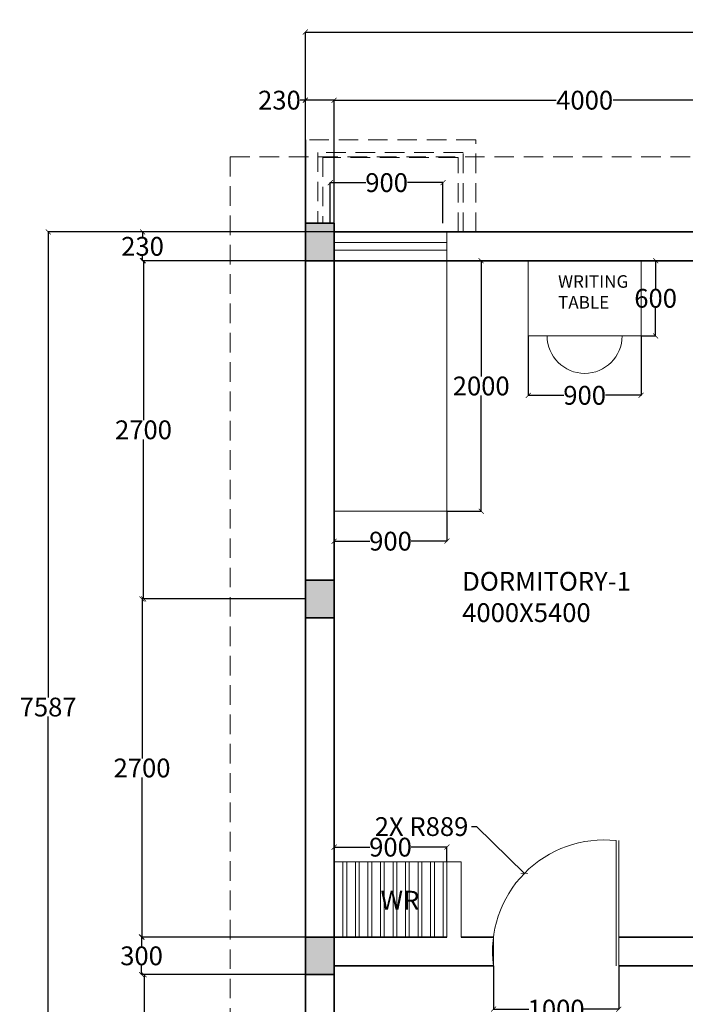
# Model space of a CAD drawing. Units: millimetres. Extents: x 32888 to 53184, y 27889 to 39696.
# Tile 2 of 6: x 32888 to 38202, y 31834 to 39696. Entities that reach past the tile are written whole.
import ezdxf

# ---------------------------------------------------------------- set-up
doc = ezdxf.new("R2010")
doc.units = ezdxf.units.MM
doc.header["$LTSCALE"] = 50
doc.header["$MEASUREMENT"] = 0
doc.linetypes.add('HIDDEN2', pattern=[0.1875, 0.125, -0.0625])
for name, color, linetype, lineweight in [('A-ANNO-DIMS', 2, 'Continuous', 18), ('A-ANNO-TEXT', 7, 'Continuous', 18), ('A-AREA-IDEN', 7, 'Continuous', 18), ('A-COLS', 1, 'Continuous', 35), ('A-COLS-PATT', 18, 'Continuous', 18), ('A-DOOR', 4, 'Continuous', 18), ('A-DOOR-HIDN', 4, 'HIDDEN2', 18), ('A-FURN', 8, 'Continuous', 18), ('A-FURN-CASE', 8, 'Continuous', 18), ('A-GLAZ', 4, 'Continuous', 18), ('A-ROOF-OVHD', 8, 'HIDDEN2', 18), ('A-WALL', 7, 'Continuous', 35)]:
    doc.layers.add(name, color=color, linetype=linetype, lineweight=lineweight)
doc.styles.get("Standard").update_dxf_attribs({"font": 'arial.ttf'})
doc.dimstyles.get("Standard").update_dxf_attribs({"dimtxt": 150, "dimasz": 40, "dimexe": 0.18, "dimexo": 0.0625, "dimgap": 0.09, "dimtad": 0, "dimtih": 1, "dimtoh": 1, "dimdec": 0, "dimzin": 0, "dimdsep": 46, "dimtxsty": 'Standard', "dimblk": 'ARCHTICK', "dimcen": 0, "dimadec": 0, "dimazin": 0, "dimtfac": 1, "dimtdec": 0, "dimtofl": 0, "dimtmove": 0, "dimatfit": 3, "dimldrblk": 'ARCHTICK', "dimfxl": 1, "dimtolj": 1, "dimtzin": 0, "dimarcsym": 1})

# ---------------------------------------------------------------- blocks, each defined once
blk = doc.blocks.new('_ArchTick')
at = {"color": 0, "linetype": 'ByBlock', "const_width": 0.15}
blk.add_lwpolyline([(-0.5, -0.5), (0.5, 0.5)], dxfattribs=at)
blk = doc.blocks.new('*D15')
at = {"layer": 'A-ANNO-DIMS', "color": 0, "lineweight": -2, "ltscale": 50, "transparency": 16777216}
for p, q in [((35398.9, 32971.1), (35398.9, 33089.1)), ((35398.9, 33088.9), (35683.4, 33088.9)), ((36298.9, 33088.9), (36014.5, 33088.9)), ((36298.9, 32971.1), (36298.9, 33089.1))]:
    blk.add_line(p, q, dxfattribs=at)
at = {"layer": 'Defpoints', "color": 0, "ltscale": 50, "transparency": 16777216}
for p in [(36298.9, 33088.9), (35398.9, 32971), (36298.9, 32971)]:
    blk.add_point(p, dxfattribs=at)
at = {"layer": 'A-ANNO-DIMS', "color": 0, "lineweight": -2, "ltscale": 50, "transparency": 16777216, "xscale": 40, "yscale": 40, "zscale": 40, "rotation": 180}
blk.add_blockref('_ArchTick', (35398.9, 33088.9), dxfattribs=at)
at = {"layer": 'A-ANNO-DIMS', "color": 0, "lineweight": -2, "ltscale": 50, "transparency": 16777216, "xscale": 40, "yscale": 40, "zscale": 40}
blk.add_blockref('_ArchTick', (36298.9, 33088.9), dxfattribs=at)
at = {"layer": 'A-ANNO-DIMS', "color": 0, "ltscale": 50, "transparency": 16777216, "insert": (35848.9, 33088.9), "char_height": 150, "attachment_point": 5}
blk.add_mtext('\\A1;900', dxfattribs=at)
blk = doc.blocks.new('*D16')
at = {"layer": 'A-ANNO-DIMS', "color": 0, "lineweight": -2, "ltscale": 50, "transparency": 16777216}
for p, q in [((36671.2, 32140.9), (36671.2, 31795.5)), ((37671.2, 32140.9), (37671.2, 31795.5)), ((36671.2, 31795.7), (36954.5, 31795.7)), ((37671.2, 31795.7), (37388, 31795.7))]:
    blk.add_line(p, q, dxfattribs=at)
at = {"layer": 'Defpoints', "color": 0, "ltscale": 50, "transparency": 16777216}
for p in [(36671.2, 32141), (37671.2, 32141), (37671.2, 31795.7)]:
    blk.add_point(p, dxfattribs=at)
at = {"layer": 'A-ANNO-DIMS', "color": 0, "lineweight": -2, "ltscale": 50, "transparency": 16777216, "xscale": 40, "yscale": 40, "zscale": 40, "rotation": 180}
blk.add_blockref('_ArchTick', (36671.2, 31795.7), dxfattribs=at)
at = {"layer": 'A-ANNO-DIMS', "color": 0, "lineweight": -2, "ltscale": 50, "transparency": 16777216, "xscale": 40, "yscale": 40, "zscale": 40}
blk.add_blockref('_ArchTick', (37671.2, 31795.7), dxfattribs=at)
at = {"layer": 'A-ANNO-DIMS', "color": 0, "ltscale": 50, "transparency": 16777216, "insert": (37171.2, 31795.7), "char_height": 150, "attachment_point": 5}
blk.add_mtext('\\A1;1000', dxfattribs=at)
blk = doc.blocks.new('*D22')
at = {"layer": 'A-ANNO-DIMS', "color": 0, "lineweight": -2, "ltscale": 50, "transparency": 16777216}
for p, q in [((35168.9, 32071), (33881.1, 32071)), ((33881.3, 32071), (33881.3, 31247.7)), ((33881.3, 30271), (33881.3, 31094.3)), ((35168.9, 30271), (33881.1, 30271))]:
    blk.add_line(p, q, dxfattribs=at)
at = {"layer": 'Defpoints', "color": 0, "ltscale": 50, "transparency": 16777216}
for p in [(35168.9, 32071), (33881.3, 30271), (35168.9, 30271)]:
    blk.add_point(p, dxfattribs=at)
at = {"layer": 'A-ANNO-DIMS', "color": 0, "lineweight": -2, "ltscale": 50, "transparency": 16777216, "xscale": 40, "yscale": 40, "zscale": 40}
for p, rotation in [((33881.3, 32071), 90), ((33881.3, 30271), 270)]:
    blk.add_blockref('_ArchTick', p, dxfattribs=dict(at, rotation=rotation))
at = {"layer": 'A-ANNO-DIMS', "color": 0, "ltscale": 50, "transparency": 16777216, "insert": (33881.3, 31171), "char_height": 150, "attachment_point": 5}
blk.add_mtext('\\A1;1800', dxfattribs=at)
blk = doc.blocks.new('*D23')
at = {"layer": 'A-ANNO-DIMS', "color": 0, "lineweight": -2, "ltscale": 50, "transparency": 16777216}
for p, q in [((35168.9, 32371), (33861.1, 32371)), ((33861.3, 32371), (33861.3, 32297.7)), ((33861.3, 32071), (33861.3, 32144.3)), ((35168.9, 32071), (33861.1, 32071))]:
    blk.add_line(p, q, dxfattribs=at)
at = {"layer": 'Defpoints', "color": 0, "ltscale": 50, "transparency": 16777216}
for p in [(33861.3, 32371), (35168.9, 32371), (35168.9, 32071)]:
    blk.add_point(p, dxfattribs=at)
at = {"layer": 'A-ANNO-DIMS', "color": 0, "lineweight": -2, "ltscale": 50, "transparency": 16777216, "xscale": 40, "yscale": 40, "zscale": 40}
for p, rotation in [((33861.3, 32371), 90), ((33861.3, 32071), 270)]:
    blk.add_blockref('_ArchTick', p, dxfattribs=dict(at, rotation=rotation))
at = {"layer": 'A-ANNO-DIMS', "color": 0, "ltscale": 50, "transparency": 16777216, "insert": (33861.3, 32221), "char_height": 150, "attachment_point": 5}
blk.add_mtext('\\A1;300', dxfattribs=at)
blk = doc.blocks.new('*D24')
at = {"layer": 'A-ANNO-DIMS', "color": 0, "lineweight": -2, "ltscale": 50, "transparency": 16777216}
for p, q in [((35168.9, 35071), (33864.9, 35071)), ((33865.1, 35071), (33865.1, 33797.7)), ((33865.1, 32371), (33865.1, 33644.3)), ((35168.9, 32371), (33864.9, 32371))]:
    blk.add_line(p, q, dxfattribs=at)
at = {"layer": 'Defpoints', "color": 0, "ltscale": 50, "transparency": 16777216}
for p in [(33865.1, 35071), (35168.9, 35071), (35168.9, 32371)]:
    blk.add_point(p, dxfattribs=at)
at = {"layer": 'A-ANNO-DIMS', "color": 0, "lineweight": -2, "ltscale": 50, "transparency": 16777216, "xscale": 40, "yscale": 40, "zscale": 40}
for p, rotation in [((33865.1, 35071), 90), ((33865.1, 32371), 270)]:
    blk.add_blockref('_ArchTick', p, dxfattribs=dict(at, rotation=rotation))
at = {"layer": 'A-ANNO-DIMS', "color": 0, "ltscale": 50, "transparency": 16777216, "insert": (33865.1, 33721), "char_height": 150, "attachment_point": 5}
blk.add_mtext('\\A1;2700', dxfattribs=at)
blk = doc.blocks.new('*D25')
at = {"layer": 'A-ANNO-DIMS', "color": 0, "lineweight": -2, "ltscale": 50, "transparency": 16777216}
for p, q in [((35168.9, 37771), (33876.5, 37771)), ((33876.7, 37771), (33876.7, 36497.7)), ((33876.7, 35071), (33876.7, 36344.3)), ((35168.9, 35071), (33876.5, 35071))]:
    blk.add_line(p, q, dxfattribs=at)
at = {"layer": 'Defpoints', "color": 0, "ltscale": 50, "transparency": 16777216}
for p in [(33876.7, 37771), (35168.9, 37771), (35168.9, 35071)]:
    blk.add_point(p, dxfattribs=at)
at = {"layer": 'A-ANNO-DIMS', "color": 0, "lineweight": -2, "ltscale": 50, "transparency": 16777216, "xscale": 40, "yscale": 40, "zscale": 40}
for p, rotation in [((33876.7, 37771), 90), ((33876.7, 35071), 270)]:
    blk.add_blockref('_ArchTick', p, dxfattribs=dict(at, rotation=rotation))
at = {"layer": 'A-ANNO-DIMS', "color": 0, "ltscale": 50, "transparency": 16777216, "insert": (33876.7, 36421), "char_height": 150, "attachment_point": 5}
blk.add_mtext('\\A1;2700', dxfattribs=at)
blk = doc.blocks.new('*D26')
at = {"layer": 'A-ANNO-DIMS', "color": 0, "lineweight": -2, "ltscale": 50, "transparency": 16777216}
for p, q in [((35398.9, 38001), (33869, 38001)), ((33869.2, 38001), (33869.2, 37962.7)), ((35398.9, 37771), (33869, 37771)), ((33869.2, 37771), (33869.2, 37809.3))]:
    blk.add_line(p, q, dxfattribs=at)
at = {"layer": 'Defpoints', "color": 0, "ltscale": 50, "transparency": 16777216}
for p in [(33869.2, 38001), (35398.9, 38001), (35398.9, 37771)]:
    blk.add_point(p, dxfattribs=at)
at = {"layer": 'A-ANNO-DIMS', "color": 0, "lineweight": -2, "ltscale": 50, "transparency": 16777216, "xscale": 40, "yscale": 40, "zscale": 40}
for p, rotation in [((33869.2, 38001), 90), ((33869.2, 37771), 270)]:
    blk.add_blockref('_ArchTick', p, dxfattribs=dict(at, rotation=rotation))
at = {"layer": 'A-ANNO-DIMS', "color": 0, "ltscale": 50, "transparency": 16777216, "insert": (33869.2, 37886), "char_height": 150, "attachment_point": 5}
blk.add_mtext('\\A1;230', dxfattribs=at)
blk = doc.blocks.new('*D39')
at = {"layer": 'A-ANNO-DIMS', "color": 0, "lineweight": -2, "ltscale": 50, "transparency": 16777216}
for p, q in [((36948.9, 37170.9), (36948.9, 36696.3)), ((37848.9, 37170.9), (37848.9, 36696.3)), ((36948.9, 36696.4), (37233.4, 36696.4)), ((37848.9, 36696.4), (37564.5, 36696.4))]:
    blk.add_line(p, q, dxfattribs=at)
at = {"layer": 'Defpoints', "color": 0, "ltscale": 50, "transparency": 16777216}
for p in [(36948.9, 37171), (37848.9, 37171), (36948.9, 36696.4)]:
    blk.add_point(p, dxfattribs=at)
at = {"layer": 'A-ANNO-DIMS', "color": 0, "lineweight": -2, "ltscale": 50, "transparency": 16777216, "xscale": 40, "yscale": 40, "zscale": 40, "rotation": 180}
blk.add_blockref('_ArchTick', (36948.9, 36696.4), dxfattribs=at)
at = {"layer": 'A-ANNO-DIMS', "color": 0, "lineweight": -2, "ltscale": 50, "transparency": 16777216, "xscale": 40, "yscale": 40, "zscale": 40}
blk.add_blockref('_ArchTick', (37848.9, 36696.4), dxfattribs=at)
at = {"layer": 'A-ANNO-DIMS', "color": 0, "ltscale": 50, "transparency": 16777216, "insert": (37398.9, 36696.4), "char_height": 150, "attachment_point": 5}
blk.add_mtext('\\A1;900', dxfattribs=at)
blk = doc.blocks.new('*D40')
at = {"layer": 'A-ANNO-DIMS', "color": 0, "lineweight": -2, "ltscale": 50, "transparency": 16777216}
for p, q in [((37849, 37771), (37965.7, 37771)), ((37965.6, 37771), (37965.6, 37547.7)), ((37965.6, 37171), (37965.6, 37394.3)), ((37849, 37171), (37965.7, 37171))]:
    blk.add_line(p, q, dxfattribs=at)
at = {"layer": 'Defpoints', "color": 0, "ltscale": 50, "transparency": 16777216}
for p in [(37848.9, 37771), (37965.6, 37771), (37848.9, 37171)]:
    blk.add_point(p, dxfattribs=at)
at = {"layer": 'A-ANNO-DIMS', "color": 0, "lineweight": -2, "ltscale": 50, "transparency": 16777216, "xscale": 40, "yscale": 40, "zscale": 40}
for p, rotation in [((37965.6, 37771), 90), ((37965.6, 37171), 270)]:
    blk.add_blockref('_ArchTick', p, dxfattribs=dict(at, rotation=rotation))
at = {"layer": 'A-ANNO-DIMS', "color": 0, "ltscale": 50, "transparency": 16777216, "insert": (37965.6, 37471), "char_height": 150, "attachment_point": 5}
blk.add_mtext('\\A1;600', dxfattribs=at)
blk = doc.blocks.new('*D41')
at = {"layer": 'A-ANNO-DIMS', "color": 0, "lineweight": -2, "ltscale": 50, "transparency": 16777216}
for p, q in [((36299, 37771), (36573.1, 37771)), ((36572.9, 37771), (36572.9, 36847.7)), ((36572.9, 35771), (36572.9, 36694.3)), ((36299, 35771), (36573.1, 35771))]:
    blk.add_line(p, q, dxfattribs=at)
at = {"layer": 'Defpoints', "color": 0, "ltscale": 50, "transparency": 16777216}
for p in [(36298.9, 37771), (36572.9, 37771), (36298.9, 35771)]:
    blk.add_point(p, dxfattribs=at)
at = {"layer": 'A-ANNO-DIMS', "color": 0, "lineweight": -2, "ltscale": 50, "transparency": 16777216, "xscale": 40, "yscale": 40, "zscale": 40}
for p, rotation in [((36572.9, 37771), 90), ((36572.9, 35771), 270)]:
    blk.add_blockref('_ArchTick', p, dxfattribs=dict(at, rotation=rotation))
at = {"layer": 'A-ANNO-DIMS', "color": 0, "ltscale": 50, "transparency": 16777216, "insert": (36572.9, 36771), "char_height": 150, "attachment_point": 5}
blk.add_mtext('\\A1;2000', dxfattribs=at)
blk = doc.blocks.new('*D42')
at = {"layer": 'A-ANNO-DIMS', "color": 0, "lineweight": -2, "ltscale": 50, "transparency": 16777216}
for p, q in [((35398.9, 35770.9), (35398.9, 35531.8)), ((36298.9, 35770.9), (36298.9, 35531.8)), ((35398.9, 35531.9), (35683.4, 35531.9)), ((36298.9, 35531.9), (36014.5, 35531.9))]:
    blk.add_line(p, q, dxfattribs=at)
at = {"layer": 'Defpoints', "color": 0, "ltscale": 50, "transparency": 16777216}
for p in [(35398.9, 35771), (36298.9, 35771), (35398.9, 35531.9)]:
    blk.add_point(p, dxfattribs=at)
at = {"layer": 'A-ANNO-DIMS', "color": 0, "lineweight": -2, "ltscale": 50, "transparency": 16777216, "xscale": 40, "yscale": 40, "zscale": 40, "rotation": 180}
blk.add_blockref('_ArchTick', (35398.9, 35531.9), dxfattribs=at)
at = {"layer": 'A-ANNO-DIMS', "color": 0, "lineweight": -2, "ltscale": 50, "transparency": 16777216, "xscale": 40, "yscale": 40, "zscale": 40}
blk.add_blockref('_ArchTick', (36298.9, 35531.9), dxfattribs=at)
at = {"layer": 'A-ANNO-DIMS', "color": 0, "ltscale": 50, "transparency": 16777216, "insert": (35848.9, 35531.9), "char_height": 150, "attachment_point": 5}
blk.add_mtext('\\A1;900', dxfattribs=at)
blk = doc.blocks.new('*D47')
at = {"layer": 'A-ANNO-DIMS', "color": 0, "lineweight": -2, "ltscale": 50, "transparency": 16777216}
for p, q in [((35367.9, 38071.1), (35367.9, 38395)), ((35367.9, 38394.8), (35652.4, 38394.8)), ((36267.9, 38394.8), (35983.5, 38394.8)), ((36267.9, 38071.1), (36267.9, 38395))]:
    blk.add_line(p, q, dxfattribs=at)
at = {"layer": 'Defpoints', "color": 0, "ltscale": 50, "transparency": 16777216}
for p in [(36267.9, 38394.8), (35367.9, 38071), (36267.9, 38071)]:
    blk.add_point(p, dxfattribs=at)
at = {"layer": 'A-ANNO-DIMS', "color": 0, "lineweight": -2, "ltscale": 50, "transparency": 16777216, "xscale": 40, "yscale": 40, "zscale": 40, "rotation": 180}
blk.add_blockref('_ArchTick', (35367.9, 38394.8), dxfattribs=at)
at = {"layer": 'A-ANNO-DIMS', "color": 0, "lineweight": -2, "ltscale": 50, "transparency": 16777216, "xscale": 40, "yscale": 40, "zscale": 40}
blk.add_blockref('_ArchTick', (36267.9, 38394.8), dxfattribs=at)
at = {"layer": 'A-ANNO-DIMS', "color": 0, "ltscale": 50, "transparency": 16777216, "insert": (35817.9, 38394.8), "char_height": 150, "attachment_point": 5}
blk.add_mtext('\\A1;900', dxfattribs=at)
blk = doc.blocks.new('*D54')
at = {"layer": 'A-ANNO-DIMS', "color": 0, "lineweight": -2, "ltscale": 50, "transparency": 16777216}
for p, q in [((35398.9, 38001.1), (35398.9, 39053.1)), ((35398.9, 39052.9), (37172.1, 39052.9)), ((39398.9, 39052.9), (37625.8, 39052.9)), ((39398.9, 38001.1), (39398.9, 39053.1))]:
    blk.add_line(p, q, dxfattribs=at)
at = {"layer": 'Defpoints', "color": 0, "ltscale": 50, "transparency": 16777216}
for p in [(35398.9, 39052.9), (35398.9, 38001), (39398.9, 38001)]:
    blk.add_point(p, dxfattribs=at)
at = {"layer": 'A-ANNO-DIMS', "color": 0, "lineweight": -2, "ltscale": 50, "transparency": 16777216, "xscale": 40, "yscale": 40, "zscale": 40, "rotation": 180}
blk.add_blockref('_ArchTick', (35398.9, 39052.9), dxfattribs=at)
at = {"layer": 'A-ANNO-DIMS', "color": 0, "lineweight": -2, "ltscale": 50, "transparency": 16777216, "xscale": 40, "yscale": 40, "zscale": 40}
blk.add_blockref('_ArchTick', (39398.9, 39052.9), dxfattribs=at)
at = {"layer": 'A-ANNO-DIMS', "color": 0, "ltscale": 50, "transparency": 16777216, "insert": (37398.9, 39052.9), "char_height": 150, "attachment_point": 5}
blk.add_mtext('\\A1;4000', dxfattribs=at)
blk = doc.blocks.new('*D55')
at = {"layer": 'A-ANNO-DIMS', "color": 0, "lineweight": -2, "ltscale": 50, "transparency": 16777216}
for p, q in [((35168.9, 39053.1), (35128.9, 39053.1)), ((35168.9, 38071.1), (35168.9, 39053.3)), ((35398.9, 39053.1), (35168.9, 39053.1)), ((35398.9, 38071.1), (35398.9, 39053.3))]:
    blk.add_line(p, q, dxfattribs=at)
at = {"layer": 'Defpoints', "color": 0, "ltscale": 50, "transparency": 16777216}
for p in [(35168.9, 39053.1), (35168.9, 38071), (35398.9, 38071)]:
    blk.add_point(p, dxfattribs=at)
at = {"layer": 'A-ANNO-DIMS', "color": 0, "lineweight": -2, "ltscale": 50, "transparency": 16777216, "xscale": 40, "yscale": 40, "zscale": 40}
for p, rotation in [((35168.9, 39053.1), 180.0000000000054), ((35398.9, 39053.1), 5.3557e-12)]:
    blk.add_blockref('_ArchTick', p, dxfattribs=dict(at, rotation=rotation))
at = {"layer": 'A-ANNO-DIMS', "color": 0, "ltscale": 50, "transparency": 16777216, "insert": (34962.1, 39053.1), "char_height": 150, "attachment_point": 5}
blk.add_mtext('\\A1;230', dxfattribs=at)
blk = doc.blocks.new('*D57')
at = {"layer": 'A-ANNO-DIMS', "color": 0, "lineweight": -2, "ltscale": 50, "transparency": 16777216}
for p, q in [((35168.9, 38001.1), (35168.9, 39597.3)), ((35168.9, 39597.2), (42753.9, 39597.2)), ((50888.9, 39597.2), (43304, 39597.2)), ((50888.9, 38001.1), (50888.9, 39597.3))]:
    blk.add_line(p, q, dxfattribs=at)
at = {"layer": 'Defpoints', "color": 0, "ltscale": 50, "transparency": 16777216}
for p in [(50888.9, 39597.2), (35168.9, 38001), (50888.9, 38001)]:
    blk.add_point(p, dxfattribs=at)
at = {"layer": 'A-ANNO-DIMS', "color": 0, "lineweight": -2, "ltscale": 50, "transparency": 16777216, "xscale": 40, "yscale": 40, "zscale": 40, "rotation": 180}
blk.add_blockref('_ArchTick', (35168.9, 39597.2), dxfattribs=at)
at = {"layer": 'A-ANNO-DIMS', "color": 0, "lineweight": -2, "ltscale": 50, "transparency": 16777216, "xscale": 40, "yscale": 40, "zscale": 40}
blk.add_blockref('_ArchTick', (50888.9, 39597.2), dxfattribs=at)
at = {"layer": 'A-ANNO-DIMS', "color": 0, "ltscale": 50, "transparency": 16777216, "insert": (43028.9, 39597.2), "char_height": 150, "attachment_point": 5}
blk.add_mtext('\\A1;15720', dxfattribs=at)
blk = doc.blocks.new('*D58')
at = {"layer": 'A-ANNO-DIMS', "color": 0, "lineweight": -2, "ltscale": 50, "transparency": 16777216}
for p, q in [((35398.9, 38001), (33115.3, 38001)), ((33115.5, 38001), (33115.5, 34284.2)), ((33115.5, 30414), (33115.5, 34130.8)), ((35398.9, 30414), (33115.3, 30414))]:
    blk.add_line(p, q, dxfattribs=at)
at = {"layer": 'Defpoints', "color": 0, "ltscale": 50, "transparency": 16777216}
for p in [(35398.9, 38001), (33115.5, 30414), (35398.9, 30414)]:
    blk.add_point(p, dxfattribs=at)
at = {"layer": 'A-ANNO-DIMS', "color": 0, "lineweight": -2, "ltscale": 50, "transparency": 16777216, "xscale": 40, "yscale": 40, "zscale": 40}
for p, rotation in [((33115.5, 38001), 90), ((33115.5, 30414), 270)]:
    blk.add_blockref('_ArchTick', p, dxfattribs=dict(at, rotation=rotation))
at = {"layer": 'A-ANNO-DIMS', "color": 0, "ltscale": 50, "transparency": 16777216, "insert": (33115.5, 34207.5), "char_height": 150, "attachment_point": 5}
blk.add_mtext('\\A1;7587', dxfattribs=at)
blk = doc.blocks.new('BED-SINGLE-900')
for p in [(900, 2230), (0, 0)]:
    blk.add_line(p, (900, 0))
blk = doc.blocks.new('DESK-WITH-CHAIR-900')
for p, q in [((0, 299.6), (0, 899.6)), ((900, 899.6), (900, 299.6)), ((900, 299.6), (0, 299.6))]:
    blk.add_line(p, q)
blk.add_arc((450, 299.6), 299.6, 180, 0)
blk = doc.blocks.new('WARDROBE-SLATTED-PANEL-900')
at = {"ltscale": 50}
for p, q in [((-830, 600), (-830, 0)), ((-800, 600), (-800, 0)), ((-730, 600), (-730, 0)), ((-700, 600), (-700, 0)), ((-630, 600), (-630, 0)), ((-600, 600), (-600, 0)), ((-530, 600), (-530, 0)), ((-500, 600), (-500, 0)), ((-430, 600), (-430, 0)), ((-400, 600), (-400, 0)), ((-330, 600), (-330, 0)), ((-300, 600), (-300, 0)), ((-230, 600), (-230, 0)), ((-200, 600), (-200, 0)), ((-130, 600), (-130, 0)), ((-100, 600), (-100, 0)), ((-30, 600), (-30, 0)), ((-30, 0), (0, 0))]:
    blk.add_line(p, q, dxfattribs=at)
blk = doc.blocks.new('DOOR-SINGLE-1000')
at = {"ltscale": 50}
for p, q in [((987.6, 0), (987.6, 1000)), ((1007.6, 0), (1007.6, 1000))]:
    blk.add_line(p, q, dxfattribs=at)
blk.add_arc((889, 116.4), 889, 83.63161, 187.52584, dxfattribs=at)
blk = doc.blocks.new('WINDOW-900')
for p, q in [((900, 60), (0, 60)), ((900, 0), (0, 0))]:
    blk.add_line(p, q)
blk = doc.blocks.new('COLUMN-IN-WALL-230x300')
for points in [[(0, 300), (230, 300)], [(230, 0), (0, 0)]]:
    blk.add_lwpolyline(points)
blk = doc.blocks.new('*D78')
at = {"layer": 'A-ANNO-DIMS', "color": 0, "lineweight": -2, "ltscale": 50, "transparency": 16777216}
for p, q in [((36496.6, 33253.1), (36536.6, 33253.1)), ((36536.6, 33253.1), (36917.6, 32879.7))]:
    blk.add_line(p, q, dxfattribs=at)
at = {"layer": 'Defpoints', "color": 0, "ltscale": 50, "transparency": 16777216}
for p in [(36917.6, 32879.7), (37552.6, 32257.5)]:
    blk.add_point(p, dxfattribs=at)
at = {"layer": 'A-ANNO-DIMS', "color": 0, "lineweight": -2, "ltscale": 50, "transparency": 16777216, "xscale": 40, "yscale": 40, "zscale": 40, "rotation": 315.5787356955544}
blk.add_blockref('_ArchTick', (36917.6, 32879.7), dxfattribs=at)
at = {"layer": 'A-ANNO-DIMS', "color": 0, "ltscale": 50, "transparency": 16777216, "insert": (36096.5, 33253.1), "char_height": 150, "attachment_point": 5}
blk.add_mtext('\\A1;2X R889', dxfattribs=at)

msp = doc.modelspace()

# ---------------------------------------------------------------- hatches: boundary and pattern name
at = {"layer": 'A-COLS-PATT', "ltscale": 50}
h = msp.add_hatch(color=256, dxfattribs=at)
h.dxf.hatch_style = 1
h.paths.add_polyline_path([(35398.95, 38071.01), (35168.95, 38071.01), (35168.95, 37771.01), (35398.95, 37771.01)])
h.paths.add_polyline_path([(39628.95, 38071.01), (39398.95, 38071.01), (39398.95, 37771.01), (39628.95, 37771.01)])
h.paths.add_polyline_path([(43903.95, 38071.01), (43673.95, 38071.01), (43673.95, 37771.01), (43903.95, 37771.01)])
h.paths.add_polyline_path([(47658.95, 38071.01), (47428.95, 38071.01), (47428.95, 37771.01), (47658.95, 37771.01)])
h.paths.add_polyline_path([(50888.95, 38071.01), (50658.95, 38071.01), (50658.95, 37771.01), (50888.95, 37771.01)])
h.paths.add_polyline_path([(50888.95, 35221.01), (50658.95, 35221.01), (50658.95, 34921.01), (50888.95, 34921.01)])
h.paths.add_polyline_path([(47658.95, 35221.01), (47428.95, 35221.01), (47428.95, 34921.01), (47658.95, 34921.01)])
h.paths.add_polyline_path([(39628.95, 35071.01), (39628.95, 35221.01), (39398.95, 35221.01), (39398.95, 34921.01), (39628.95, 34921.01)])
h.paths.add_polyline_path([(35398.95, 35221.01), (35168.95, 35221.01), (35168.95, 34921.01), (35398.95, 34921.01)])
h.paths.add_polyline_path([(35398.95, 32371.01), (35168.95, 32371.01), (35168.95, 32071.01), (35398.95, 32071.01)])
h.paths.add_polyline_path([(35418.95, 30571.01), (35168.95, 30571.01), (35168.95, 30271.01), (35418.95, 30271.01)])
h.paths.add_polyline_path([(39642.61, 30571.01), (39392.61, 30571.01), (39392.61, 30271.01), (39642.61, 30271.01)])
h.paths.add_polyline_path([(39628.95, 32371.01), (39398.95, 32371.01), (39398.95, 32071.01), (39628.95, 32071.01)])
h.paths.add_polyline_path([(43903.95, 32371.01), (43673.95, 32371.01), (43673.95, 32071.01), (43903.95, 32071.01)])
h.paths.add_polyline_path([(43903.95, 30571.01), (43653.95, 30571.01), (43653.95, 30271.01), (43903.95, 30271.01)])
h.paths.add_polyline_path([(47658.95, 32441.01), (47428.95, 32441.01), (47428.95, 32141.01), (47658.95, 32141.01)])
h.paths.add_polyline_path([(50888.95, 32414.45), (50658.95, 32414.45), (50658.95, 32114.45), (50888.95, 32114.45)])
h.paths.add_polyline_path([(50888.95, 30571.01), (50638.95, 30571.01), (50638.95, 30271.01), (50888.95, 30271.01)])
h.paths.add_polyline_path([(47678.95, 30571.01), (47428.95, 30571.01), (47428.95, 30341.01), (47678.95, 30341.01)])
h.paths.add_polyline_path([(47678.95, 30341.01), (47428.95, 30341.01), (47428.95, 30271.01), (47678.95, 30271.01)])

# ---------------------------------------------------------------- linework, layer by layer
at = {"layer": 'A-COLS'}
for points in [[(35398.95, 38071.01), (35168.95, 38071.01)], [(35398.95, 32071.01), (35168.95, 32071.01)]]:
    msp.add_lwpolyline(points, dxfattribs=at)
at = {"layer": 'A-DOOR-HIDN', "ltscale": 50}
for p, q in [((36671.2, 32141.01), (36671.2, 32371.01)), ((37671.2, 32371.01), (37671.2, 32141.01))]:
    msp.add_line(p, q, dxfattribs=at)
at = {"layer": 'A-FURN-CASE', "ltscale": 50}
for p, q in [((36413.95, 32971.01), (35398.95, 32971.01)), ((36298.95, 32971.01), (36298.95, 32371.01)), ((36413.95, 32971.01), (36413.95, 32371.01))]:
    msp.add_line(p, q, dxfattribs=at)
at = {"layer": 'A-ROOF-OVHD', "ltscale": 25}
for q in [(51488.95, 38601.01), (34568.95, 29741.01)]:
    msp.add_line((34568.95, 38601.01), q, dxfattribs=at)
for points in [[(36528.95, 38001.01), (36528.95, 38736.01), (35168.95, 38736.01)], [(36428.95, 38001.01), (36428.95, 38636.01), (35268.95, 38636.01), (35268.95, 38071.01)], [(36388.95, 38001.01), (36388.95, 38596.01), (35308.95, 38596.01), (35308.95, 38071.01)]]:
    msp.add_lwpolyline(points, dxfattribs=at)
at = {"layer": 'A-WALL'}
for p, q in [((35168.95, 38736.01), (35168.95, 30271.01)), ((35398.95, 38071.01), (35398.95, 30571.01)), ((35398.95, 38001.01), (39398.95, 38001.01)), ((36298.95, 32371.01), (35168.95, 32371.01)), ((36413.95, 32371.01), (36671.2, 32371.01)), ((37671.2, 32371.01), (38383.95, 32371.01)), ((35398.95, 32141.01), (36671.2, 32141.01)), ((37671.2, 32141.01), (39398.95, 32141.01))]:
    msp.add_line(p, q, dxfattribs=at)
msp.add_lwpolyline([(35168.95, 37771.01), (41123.95, 37771.01)], dxfattribs=at)

# ---------------------------------------------------------------- block references
at = {"layer": 'A-COLS'}
msp.add_blockref('COLUMN-IN-WALL-230x300', (35168.95, 34921.01), dxfattribs=at)
at = {"layer": 'A-DOOR'}
msp.add_blockref('DOOR-SINGLE-1000', (36663.6, 32141.01), dxfattribs=at)
at = {"layer": 'A-FURN'}
for name, p in [('BED-SINGLE-900', (35398.95, 35771.01)), ('DESK-WITH-CHAIR-900', (36948.95, 36871.43))]:
    msp.add_blockref(name, p, dxfattribs=at)
at = {"layer": 'A-FURN-CASE'}
msp.add_blockref('WARDROBE-SLATTED-PANEL-900', (36298.95, 32371.01), dxfattribs=at)
at = {"layer": 'A-GLAZ'}
msp.add_blockref('WINDOW-900', (35398.95, 37856.01), dxfattribs=at)

# ---------------------------------------------------------------- texts
at = {"layer": 'A-ANNO-TEXT', "ltscale": 50, "attachment_point": 1}
for s, width, insert, char_height in [('WRITING\\PTABLE', 901.3249, (37186.5, 37655.34), 100), ('WR', 742.516, (35768.95, 32740.14), 150)]:
    msp.add_mtext_dynamic_manual_height_columns(s, width=width, gutter_width=1, heights=[0], dxfattribs=dict(at, insert=insert, char_height=char_height))
at = {"layer": 'A-AREA-IDEN', "ltscale": 50, "insert": (36421.25, 35286.3), "char_height": 150, "attachment_point": 1}
msp.add_mtext_dynamic_manual_height_columns('DORMITORY-1\\P4000X5400', width=901.3249, gutter_width=1, heights=[0], dxfattribs=at)

# ---------------------------------------------------------------- dimensions: what is measured, and where the dimension line sits
at = {"layer": 'A-ANNO-DIMS', "ltscale": 50}
for p1, p2, distance, picture, middle in [((35168.95, 38001.01), (50888.95, 38001.01), 1596.15, '*D57', (43028.95, 39597.16)), ((35398.95, 38071.01), (35168.95, 38071.01), -982.08, '*D55', (34962.13, 39053.09)), ((39398.95, 38001.01), (35398.95, 38001.01), -1051.9, '*D54', (37398.95, 39052.91)), ((35367.95, 38071.01), (36267.95, 38071.01), 323.79, '*D47', (35817.95, 38394.8)), ((35398.95, 38001.01), (35398.95, 30414.01), -2283.42, '*D58', (33115.53, 34207.51)), ((35398.95, 37771.01), (35398.95, 38001.01), 1529.78, '*D26', (33869.17, 37886.01)), ((35168.95, 35071.01), (35168.95, 37771.01), 1292.24, '*D25', (33876.71, 36421.01)), ((36298.95, 35771.01), (36298.95, 37771.01), -273.93, '*D41', (36572.88, 36771.01)), ((37848.95, 37171.01), (37848.95, 37771.01), -116.6, '*D40', (37965.55, 37471.01)), ((37848.95, 37171.01), (36948.95, 37171.01), 474.56, '*D39', (37398.95, 36696.45)), ((36298.95, 35771.01), (35398.95, 35771.01), 239.06, '*D42', (35848.95, 35531.95)), ((35168.95, 32371.01), (35168.95, 35071.01), 1303.88, '*D24', (33865.07, 33721.01)), ((35398.95, 32971.01), (36298.95, 32971.01), 117.89, '*D15', (35848.95, 33088.9)), ((35168.95, 32071.01), (35168.95, 32371.01), 1307.67, '*D23', (33861.28, 32221.01)), ((35168.95, 32071.01), (35168.95, 30271.01), -1287.67, '*D22', (33881.28, 31171.01)), ((36671.2, 32141.01), (37671.2, 32141.01), -345.35, '*D16', (37171.2, 31795.66))]:
    dim = msp.add_aligned_dim(p1=p1, p2=p2, distance=distance, dimstyle='Standard', override={"dimclrd": 0, "dimclre": 0, "dimclrt": 0}, dxfattribs=at)
    dim.commit()
    dim.dimension.update_dxf_attribs({"geometry": picture, "text_midpoint": middle})
dim = msp.add_radius_dim(center=(37552.59, 32257.45), mpoint=(36917.62, 32879.72), text='2X <>', dimstyle='Standard', override={"dimdec": 0, "dimlfac": 1, "dimrnd": 0, "dimzin": 0, "dimdsep": 46, "dimlunit": 2}, dxfattribs=at)
dim.commit()
dim.dimension.update_dxf_attribs({"geometry": '*D78', "text_midpoint": (36096.48, 33253.08), "dimtype": 164})

doc.saveas('drawing.dxf')
